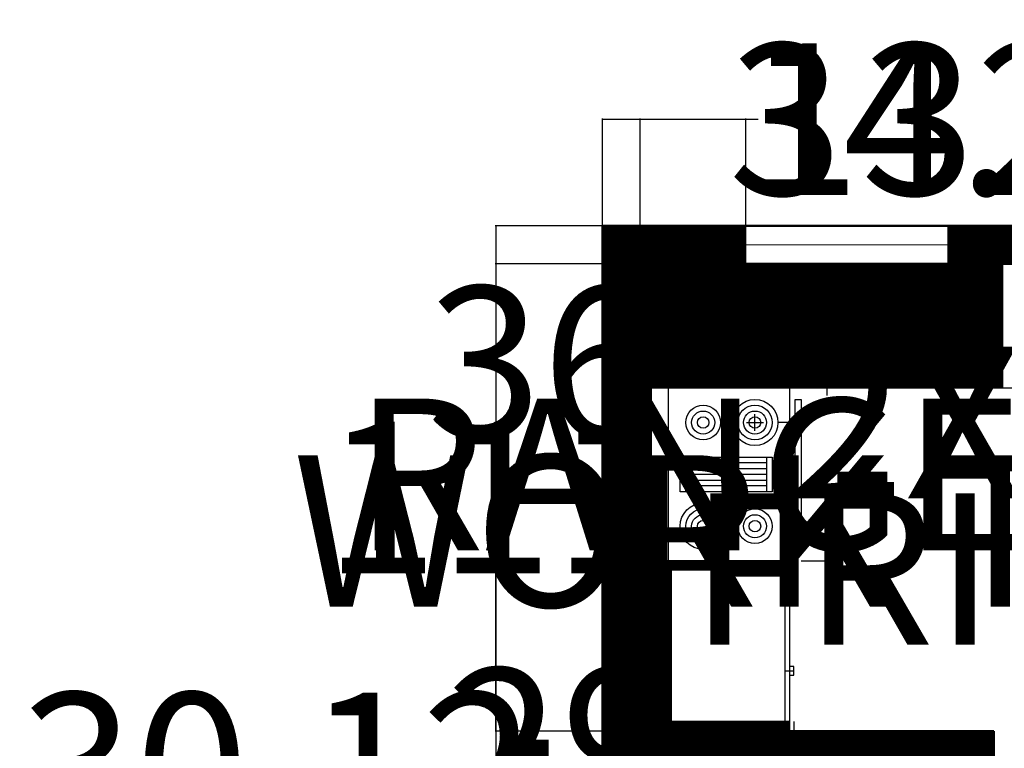
# Model space of a CAD drawing. Units: inches. Extents: x 1173 to 2157, y 515 to 1129.
# Tile 3 of 13: x 1241 to 1475, y 929 to 1102. Entities that reach past the tile are written whole.
import ezdxf

# ---------------------------------------------------------------- set-up
doc = ezdxf.new("R2010")
doc.units = ezdxf.units.IN
doc.header["$MEASUREMENT"] = 0
for name, color, linetype, lineweight in [('A-ANNO-DIMS', 2, 'Continuous', 18), ('A-EQPM', 9, 'Continuous', 25), ('A-FLOR-CASE', 32, 'Continuous', 25), ('A-GLAZ', 4, 'Continuous', 18), ('A-WALL', 7, 'Continuous', 50)]:
    doc.layers.add(name, color=color, linetype=linetype, lineweight=lineweight)
doc.layers.add('A-FLOR-CASE-PATT', color=28, linetype='Continuous', lineweight=13, true_color=0x301203)
doc.layers.add('A-WALL-PATT', color=22, linetype='Continuous', lineweight=13, true_color=0xca4b0c)
doc.styles.get("Standard").update_dxf_attribs({"font": 'arial.ttf'})
doc.dimstyles.get("Standard").update_dxf_attribs({"dimtxt": 36, "dimasz": 0.18, "dimexe": 0.18, "dimexo": 0.0625, "dimgap": 0.09, "dimtad": 0, "dimtih": 1, "dimtoh": 1, "dimdec": 0, "dimrnd": 72, "dimzin": 0, "dimdsep": 46, "dimlunit": 3, "dimtxsty": 'Standard', "dimcen": 2, "dimadec": 0, "dimazin": 0, "dimtfac": 1, "dimtdec": 0, "dimtofl": 0, "dimtmove": 0, "dimatfit": 3, "dimfxl": 1, "dimtolj": 1, "dimtzin": 0, "dimarcsym": 0})

# ---------------------------------------------------------------- blocks, each defined once
blk = doc.blocks.new('Range-Oven - 30 in top')
for p, q in [((0, -3), (30, -3)), ((12, -6), (18, -6)), ((13, -20), (13, -6)), ((14, -6), (14, -20)), ((15, -20), (15, -6)), ((16, -6), (16, -20)), ((17, -20), (17, -6)), ((18, -20), (12, -20)), ((6, -24), (6, -25)), ((8, -25), (8, -24)), ((22, -25), (22, -24)), ((24, -24), (24, -25))]:
    blk.add_line(p, q)
for points in [[(0, -24), (0, 0), (30, 0), (30, -24)], [(12, -21), (12, -5), (18, -5), (18, -21)], [(2, -26), (2, -25), (28, -25), (28, -26)]]:
    blk.add_lwpolyline(points, close=True)
for centre, radius in [((6, -9), 4), ((6, -9), 3), ((24, -9), 3), ((6, -9), 2), ((6, -9), 1), ((24, -9), 2), ((24, -9), 1), ((6, -18), 3), ((24, -18), 4), ((24, -18), 3), ((6, -18), 2), ((6, -18), 1), ((24, -18), 2), ((24, -18), 1)]:
    blk.add_circle(centre, radius)
blk = doc.blocks.new('Refrigerator-2 door - 36 in top')
for p, q in [((0, -26.999999), (36, -26.999999)), ((11, -27.999999), (11, -28.999999)), ((12, -26.999999), (12, -28.999999)), ((13, -28.999999), (13, -27.999999)), ((11, -28.999999), (13, -28.999999))]:
    blk.add_line(p, q)
blk.add_lwpolyline([(0, -27.999999), (0, 0), (36, 0), (36, -27.999999)], close=True)
blk = doc.blocks.new('WIN-48X9')
blk.add_line((48, 4.5), (0, 4.5))
blk.add_lwpolyline([(0, 9), (48, 9), (48, 0), (0, 0)], close=True)
blk = doc.blocks.new('*D36')
at = {"layer": 'A-ANNO-DIMS', "color": 0, "lineweight": -2, "transparency": 16777216}
for p, q in [((1497.87, 905.02), (1487.37, 905.02)), ((1487.55, 904.84), (1487.55, 889.09)), ((1487.55, 835.93), (1487.55, 851.68)), ((1497.87, 835.75), (1487.37, 835.75))]:
    blk.add_line(p, q, dxfattribs=at)
at = {"layer": 'A-ANNO-DIMS', "color": 0, "transparency": 16777216}
for points in [[(1487.52, 904.84), (1487.58, 904.84), (1487.55, 905.02)], [(1487.52, 835.93), (1487.58, 835.93), (1487.55, 835.75)]]:
    blk.add_solid(points, dxfattribs=at)
at = {"layer": 'Defpoints', "color": 0, "transparency": 16777216}
for p in [(1497.94, 905.02), (1487.55, 835.75), (1497.94, 835.75)]:
    blk.add_point(p, dxfattribs=at)
at = {"layer": 'A-ANNO-DIMS', "color": 0, "transparency": 16777216, "insert": (1487.55, 870.38), "char_height": 36, "attachment_point": 5}
blk.add_mtext('\\A1;DINING SET 69', dxfattribs=at)
blk = doc.blocks.new('*D46')
at = {"layer": 'A-ANNO-DIMS', "color": 0, "lineweight": -2, "transparency": 16777216}
for p, q in [((1646.37, 911.98), (1645.86, 896.32)), ((1648.72, 912.09), (1646.2, 912.17)), ((1648.2, 896.07), (1645.68, 896.15)), ((1645.86, 896.14), (1645.85, 895.96)), ((1645.85, 895.96), (1645.67, 895.96))]:
    blk.add_line(p, q, dxfattribs=at)
at = {"layer": 'A-ANNO-DIMS', "color": 0, "transparency": 16777216}
for points in [[(1646.34, 911.99), (1646.4, 911.98), (1646.38, 912.16)], [(1645.83, 896.32), (1645.89, 896.32), (1645.86, 896.14)]]:
    blk.add_solid(points, dxfattribs=at)
at = {"layer": 'Defpoints', "color": 0, "transparency": 16777216}
for p in [(1648.78, 912.09), (1645.86, 896.14), (1648.26, 896.06)]:
    blk.add_point(p, dxfattribs=at)
at = {"layer": 'A-ANNO-DIMS', "color": 0, "transparency": 16777216, "insert": (1538.16, 895.96), "char_height": 36, "attachment_point": 5}
blk.add_mtext('\\A1;BASIN 16', dxfattribs=at)
blk = doc.blocks.new('*D54')
at = {"layer": 'A-ANNO-DIMS', "color": 0, "lineweight": -2, "transparency": 16777216}
for p, q in [((1496.35, 1005.18), (1488.93, 1005.18)), ((1489.11, 1005), (1489.11, 999.54)), ((1489.11, 956.65), (1489.11, 962.11)), ((1496.35, 956.47), (1488.93, 956.47))]:
    blk.add_line(p, q, dxfattribs=at)
at = {"layer": 'A-ANNO-DIMS', "color": 0, "transparency": 16777216}
for points in [[(1489.08, 1005), (1489.14, 1005), (1489.11, 1005.18)], [(1489.08, 956.65), (1489.14, 956.65), (1489.11, 956.47)]]:
    blk.add_solid(points, dxfattribs=at)
at = {"layer": 'Defpoints', "color": 0, "transparency": 16777216}
for p in [(1496.42, 1005.18), (1489.11, 956.47), (1496.42, 956.47)]:
    blk.add_point(p, dxfattribs=at)
at = {"layer": 'A-ANNO-DIMS', "color": 0, "transparency": 16777216, "insert": (1489.11, 980.83), "char_height": 36, "attachment_point": 5}
blk.add_mtext('\\A1;WORK TABLE 49', dxfattribs=at)
blk = doc.blocks.new('*D56')
at = {"layer": 'A-ANNO-DIMS', "color": 0, "lineweight": -2, "transparency": 16777216}
for p, q in [((1426.92, 1014.79), (1433.2, 1014.79)), ((1433.02, 1014.61), (1433.02, 1012.98)), ((1426.92, 973.76), (1433.2, 973.76)), ((1433.02, 973.94), (1433.02, 975.57))]:
    blk.add_line(p, q, dxfattribs=at)
at = {"layer": 'A-ANNO-DIMS', "color": 0, "transparency": 16777216}
for points in [[(1432.99, 1014.61), (1433.05, 1014.61), (1433.02, 1014.79)], [(1432.99, 973.94), (1433.05, 973.94), (1433.02, 973.76)]]:
    blk.add_solid(points, dxfattribs=at)
at = {"layer": 'Defpoints', "color": 0, "transparency": 16777216}
for p in [(1426.86, 1014.79), (1433.02, 1014.79), (1426.86, 973.76)]:
    blk.add_point(p, dxfattribs=at)
at = {"layer": 'A-ANNO-DIMS', "color": 0, "transparency": 16777216, "insert": (1433.02, 994.27), "char_height": 36, "attachment_point": 5}
blk.add_mtext('\\A1;RANGE 41', dxfattribs=at)
blk = doc.blocks.new('*D57')
at = {"layer": 'A-ANNO-DIMS', "color": 0, "lineweight": -2, "transparency": 16777216}
for p, q in [((1391.3, 1020.94), (1391.12, 1020.94)), ((1391.3, 1014.85), (1391.3, 1021.12)), ((1426.68, 1020.94), (1391.48, 1020.94)), ((1426.86, 1014.85), (1426.86, 1021.12))]:
    blk.add_line(p, q, dxfattribs=at)
at = {"layer": 'A-ANNO-DIMS', "color": 0, "transparency": 16777216}
for points in [[(1391.48, 1020.97), (1391.48, 1020.91), (1391.3, 1020.94)], [(1426.68, 1020.97), (1426.68, 1020.91), (1426.86, 1020.94)]]:
    blk.add_solid(points, dxfattribs=at)
at = {"layer": 'Defpoints', "color": 0, "transparency": 16777216}
for p in [(1391.3, 1020.94), (1391.3, 1014.79), (1426.86, 1014.79)]:
    blk.add_point(p, dxfattribs=at)
at = {"layer": 'A-ANNO-DIMS', "color": 0, "transparency": 16777216, "insert": (1365.27, 1020.94), "char_height": 36, "attachment_point": 5}
blk.add_mtext('\\A1;36', dxfattribs=at)
blk = doc.blocks.new('*D60')
at = {"layer": 'A-ANNO-DIMS', "color": 0, "lineweight": -2, "transparency": 16777216}
for p, q in [((1396.06, 971.62), (1390.55, 971.62)), ((1390.73, 971.62), (1390.73, 971.8)), ((1390.73, 971.8), (1390.91, 971.8)), ((1390.73, 935.8), (1390.73, 971.44)), ((1396.06, 935.62), (1390.55, 935.62))]:
    blk.add_line(p, q, dxfattribs=at)
at = {"layer": 'A-ANNO-DIMS', "color": 0, "transparency": 16777216}
for points in [[(1390.7, 971.44), (1390.76, 971.44), (1390.73, 971.62)], [(1390.7, 935.8), (1390.76, 935.8), (1390.73, 935.62)]]:
    blk.add_solid(points, dxfattribs=at)
at = {"layer": 'Defpoints', "color": 0, "transparency": 16777216}
for p in [(1390.73, 971.62), (1396.13, 971.62), (1396.13, 935.62)]:
    blk.add_point(p, dxfattribs=at)
at = {"layer": 'A-ANNO-DIMS', "color": 0, "transparency": 16777216, "insert": (1517.73, 971.8), "char_height": 36, "attachment_point": 5}
blk.add_mtext('\\A1;FRIDGE 36', dxfattribs=at)
blk = doc.blocks.new('*D61')
at = {"layer": 'A-ANNO-DIMS', "color": 0, "lineweight": -2, "transparency": 16777216}
for p, q in [((1396.13, 935.56), (1396.13, 930.04)), ((1425.13, 935.56), (1425.13, 930.04)), ((1396.13, 930.22), (1395.95, 930.22)), ((1424.95, 930.22), (1396.31, 930.22))]:
    blk.add_line(p, q, dxfattribs=at)
at = {"layer": 'A-ANNO-DIMS', "color": 0, "transparency": 16777216}
for points in [[(1396.31, 930.25), (1396.31, 930.19), (1396.13, 930.22)], [(1424.95, 930.25), (1424.95, 930.19), (1425.13, 930.22)]]:
    blk.add_solid(points, dxfattribs=at)
at = {"layer": 'Defpoints', "color": 0, "transparency": 16777216}
for p in [(1396.13, 935.62), (1425.13, 935.62), (1396.13, 930.22)]:
    blk.add_point(p, dxfattribs=at)
at = {"layer": 'A-ANNO-DIMS', "color": 0, "transparency": 16777216, "insert": (1369.73, 930.22), "char_height": 36, "attachment_point": 5}
blk.add_mtext('\\A1;29', dxfattribs=at)
blk = doc.blocks.new('*D65')
at = {"layer": 'A-ANNO-DIMS', "color": 0, "lineweight": -2, "transparency": 16777216}
for p, q in [((1379.6, 1053.28), (1354.18, 1053.28)), ((1354.36, 1053.1), (1354.36, 827.25)), ((1354.36, 564.46), (1354.36, 790.31)), ((1379.6, 564.28), (1354.18, 564.28))]:
    blk.add_line(p, q, dxfattribs=at)
at = {"layer": 'A-ANNO-DIMS', "color": 0, "transparency": 16777216}
for points in [[(1354.33, 1053.1), (1354.39, 1053.1), (1354.36, 1053.28)], [(1354.33, 564.46), (1354.39, 564.46), (1354.36, 564.28)]]:
    blk.add_solid(points, dxfattribs=at)
at = {"layer": 'Defpoints', "color": 0, "transparency": 16777216}
for p in [(1354.36, 1053.28), (1379.66, 1053.28), (1379.66, 564.28)]:
    blk.add_point(p, dxfattribs=at)
at = {"layer": 'A-ANNO-DIMS', "color": 0, "transparency": 16777216, "insert": (1354.36, 808.78), "char_height": 36, "attachment_point": 5}
blk.add_mtext('\\A1;489', dxfattribs=at)
blk = doc.blocks.new('*D66')
at = {"layer": 'A-ANNO-DIMS', "color": 0, "lineweight": -2, "transparency": 16777216}
for p, q in [((1388.6, 1044.28), (1354.18, 1044.28)), ((1354.36, 1044.1), (1354.36, 1006.94)), ((1354.36, 933.46), (1354.36, 970.62)), ((1388.6, 933.28), (1354.18, 933.28))]:
    blk.add_line(p, q, dxfattribs=at)
at = {"layer": 'A-ANNO-DIMS', "color": 0, "transparency": 16777216}
for points in [[(1354.33, 1044.1), (1354.39, 1044.1), (1354.36, 1044.28)], [(1354.33, 933.46), (1354.39, 933.46), (1354.36, 933.28)]]:
    blk.add_solid(points, dxfattribs=at)
at = {"layer": 'Defpoints', "color": 0, "transparency": 16777216}
for p in [(1354.36, 1044.28), (1388.66, 1044.28), (1388.66, 933.28)]:
    blk.add_point(p, dxfattribs=at)
at = {"layer": 'A-ANNO-DIMS', "color": 0, "transparency": 16777216, "insert": (1354.36, 988.78), "char_height": 36, "attachment_point": 5}
blk.add_mtext('\\A1;111', dxfattribs=at)
blk = doc.blocks.new('*D67')
at = {"layer": 'A-ANNO-DIMS', "color": 0, "lineweight": -2, "transparency": 16777216}
for p, q in [((1388.66, 1044.34), (1388.66, 1078.79)), ((1388.84, 1078.61), (1416.68, 1078.61)), ((1520.48, 1078.61), (1492.64, 1078.61)), ((1520.66, 1044.34), (1520.66, 1078.79))]:
    blk.add_line(p, q, dxfattribs=at)
at = {"layer": 'A-ANNO-DIMS', "color": 0, "transparency": 16777216}
for points in [[(1388.84, 1078.64), (1388.84, 1078.58), (1388.66, 1078.61)], [(1520.48, 1078.64), (1520.48, 1078.58), (1520.66, 1078.61)]]:
    blk.add_solid(points, dxfattribs=at)
at = {"layer": 'Defpoints', "color": 0, "transparency": 16777216}
for p in [(1520.66, 1078.61), (1388.66, 1044.28), (1520.66, 1044.28)]:
    blk.add_point(p, dxfattribs=at)
at = {"layer": 'A-ANNO-DIMS', "color": 0, "transparency": 16777216, "insert": (1454.66, 1078.61), "char_height": 36, "attachment_point": 5}
blk.add_mtext('\\A1;132', dxfattribs=at)
blk = doc.blocks.new('*D68')
at = {"layer": 'A-ANNO-DIMS', "color": 0, "lineweight": -2, "transparency": 16777216}
for p, q in [((1379.66, 1053.34), (1379.66, 1078.79)), ((1379.84, 1078.61), (1413.58, 1078.61)), ((1413.76, 1053.34), (1413.76, 1078.79)), ((1413.76, 1078.61), (1413.94, 1078.61))]:
    blk.add_line(p, q, dxfattribs=at)
at = {"layer": 'A-ANNO-DIMS', "color": 0, "transparency": 16777216}
for points in [[(1379.84, 1078.64), (1379.84, 1078.58), (1379.66, 1078.61)], [(1413.58, 1078.64), (1413.58, 1078.58), (1413.76, 1078.61)]]:
    blk.add_solid(points, dxfattribs=at)
at = {"layer": 'Defpoints', "color": 0, "transparency": 16777216}
for p in [(1413.76, 1078.61), (1379.66, 1053.28), (1413.76, 1053.28)]:
    blk.add_point(p, dxfattribs=at)
at = {"layer": 'A-ANNO-DIMS', "color": 0, "transparency": 16777216, "insert": (1457.3, 1078.61), "char_height": 36, "attachment_point": 5}
blk.add_mtext('\\A1;34.1', dxfattribs=at)
blk = doc.blocks.new('*D82')
at = {"layer": 'A-ANNO-DIMS', "color": 0, "lineweight": -2, "transparency": 16777216}
for p, q in [((1363.36, 924.45), (1363.18, 924.45)), ((1388.6, 924.28), (1363.18, 924.27)), ((1363.36, 924.27), (1363.36, 924.45)), ((1363.38, 894.33), (1363.36, 924.09)), ((1388.62, 894.16), (1363.2, 894.15))]:
    blk.add_line(p, q, dxfattribs=at)
at = {"layer": 'A-ANNO-DIMS', "color": 0, "transparency": 16777216}
for points in [[(1363.39, 924.09), (1363.33, 924.09), (1363.36, 924.27)], [(1363.41, 894.33), (1363.35, 894.33), (1363.38, 894.15)]]:
    blk.add_solid(points, dxfattribs=at)
at = {"layer": 'Defpoints', "color": 0, "transparency": 16777216}
for p in [(1363.36, 924.27), (1388.66, 924.28), (1388.68, 894.16)]:
    blk.add_point(p, dxfattribs=at)
at = {"layer": 'A-ANNO-DIMS', "color": 0, "transparency": 16777216, "insert": (1302.55, 924.45), "char_height": 36, "attachment_point": 5}
blk.add_mtext('\\A1;30.12', dxfattribs=at)
blk = doc.blocks.new('*D93')
at = {"layer": 'A-ANNO-DIMS', "color": 0, "lineweight": -2, "transparency": 16777216}
for p, q in [((1473.15, 924.28), (1498.57, 924.28)), ((1498.39, 924.1), (1498.39, 913.61)), ((1473.15, 913.43), (1498.57, 913.43)), ((1498.39, 913.25), (1498.21, 913.25)), ((1498.39, 913.43), (1498.39, 913.25))]:
    blk.add_line(p, q, dxfattribs=at)
at = {"layer": 'A-ANNO-DIMS', "color": 0, "transparency": 16777216}
for points in [[(1498.36, 924.1), (1498.42, 924.1), (1498.39, 924.28)], [(1498.36, 913.61), (1498.42, 913.61), (1498.39, 913.43)]]:
    blk.add_solid(points, dxfattribs=at)
at = {"layer": 'Defpoints', "color": 0, "transparency": 16777216}
for p in [(1473.08, 924.28), (1473.08, 913.43), (1498.39, 913.43)]:
    blk.add_point(p, dxfattribs=at)
at = {"layer": 'A-ANNO-DIMS', "color": 0, "transparency": 16777216, "insert": (1425.05, 913.25), "char_height": 36, "attachment_point": 5}
blk.add_mtext('\\A1;10.848', dxfattribs=at)
blk = doc.blocks.new('*D109')
at = {"layer": 'A-ANNO-DIMS', "color": 0, "lineweight": -2, "transparency": 16777216}
for p, q in [((1638.72, 893.14), (1638.9, 893.14)), ((1638.9, 893.14), (1639.74, 886.91)), ((1641.2, 874.07), (1641.2, 878.07)), ((1639.2, 876.07), (1643.2, 876.07))]:
    blk.add_line(p, q, dxfattribs=at)
at = {"layer": 'A-ANNO-DIMS', "color": 0, "transparency": 16777216}
blk.add_solid([(1639.77, 886.92), (1639.71, 886.91), (1639.77, 886.74)], dxfattribs=at)
at = {"layer": 'Defpoints', "color": 0, "transparency": 16777216}
for p in [(1639.77, 886.74), (1641.2, 876.07)]:
    blk.add_point(p, dxfattribs=at)
at = {"layer": 'A-ANNO-DIMS', "color": 0, "transparency": 16777216, "insert": (1507.71, 893.14), "char_height": 36, "attachment_point": 5}
blk.add_mtext('\\A1;2X R10.766', dxfattribs=at)
blk = doc.blocks.new('*D110')
at = {"layer": 'A-ANNO-DIMS', "color": 0, "lineweight": -2, "transparency": 16777216}
for p, q in [((1415.92, 1004.58), (1415.92, 1008.58)), ((1413.92, 1006.58), (1417.92, 1006.58)), ((1424.67, 1006.58), (1421.57, 1006.58))]:
    blk.add_line(p, q, dxfattribs=at)
at = {"layer": 'A-ANNO-DIMS', "color": 0, "transparency": 16777216}
blk.add_solid([(1421.57, 1006.61), (1421.57, 1006.55), (1421.39, 1006.58)], dxfattribs=at)
at = {"layer": 'Defpoints', "color": 0, "transparency": 16777216}
for p in [(1410.45, 1006.58), (1421.39, 1006.58)]:
    blk.add_point(p, dxfattribs=at)
at = {"layer": 'A-ANNO-DIMS', "color": 0, "transparency": 16777216, "insert": (1556.91, 1006.58), "char_height": 36, "attachment_point": 5}
blk.add_mtext('\\A1;2X ∅10.942', dxfattribs=at)

msp = doc.modelspace()

# ---------------------------------------------------------------- hatches: boundary and pattern name
at = {"layer": 'A-FLOR-CASE-PATT'}
h = msp.add_hatch(dxfattribs=at)
h.set_pattern_fill('ANSI31', color=256)
h.paths.add_polyline_path([(1474.7462, 1044.2805), (1388.6635, 1044.2805), (1388.6635, 1014.7866), (1474.7462, 1014.7866)])
h.paths.add_polyline_path([(1396.1251, 971.618), (1424.1251, 971.618), (1424.1251, 973.7559), (1391.3005, 973.7559), (1391.3005, 1014.7866), (1388.6635, 1014.7866), (1388.6635, 933.2805), (1424.1251, 933.2805), (1424.1251, 935.618), (1396.1251, 935.618)])
at = {"layer": 'A-WALL-PATT'}
h = msp.add_hatch(dxfattribs=at)
h.set_pattern_fill('ANSI31', color=256)
h.paths.add_polyline_path([(1388.6635, 933.2805), (1388.6635, 1044.2805), (1413.7618, 1044.2805), (1413.7618, 1053.2805), (1379.6635, 1053.2805), (1379.6635, 894.1606), (1388.6635, 894.1606), (1388.6635, 924.2805), (1472.6635, 924.2805), (1472.6635, 933.2805)])
h.paths.add_polyline_path([(1520.6635, 1044.2805), (1520.6635, 1014.7866), (1520.6635, 1005.1794), (1520.7714, 1005.1794), (1520.7714, 956.4707), (1520.6635, 924.2805), (1529.6635, 924.2805), (1529.6635, 931.4788), (1529.6635, 1044.2805), (1530.8474, 1044.2805), (1570.9543, 1044.2805), (1570.9543, 1053.2805), (1461.7618, 1053.2805), (1461.7618, 1044.2805)])
h.paths.add_polyline_path([(1618.9543, 1053.2805), (1618.9543, 1044.2805), (1661.6635, 1044.2805), (1661.6635, 1043.7367), (1661.6635, 1032.8874), (1670.6635, 1032.8874), (1670.6635, 1053.2805)])
h.paths.add_polyline_path([(1661.6635, 933.2805), (1661.6635, 927.8377), (1661.6635, 924.2805), (1661.6635, 918.9156), (1670.6635, 918.9156), (1670.6635, 984.8874), (1661.6635, 984.8874), (1661.6635, 978.3712)])
h.paths.add_polyline_path([(1670.6635, 894.9156), (1661.6635, 894.9156), (1661.6635, 890.0349), (1661.9328, 890.0349), (1661.9328, 870.079), (1661.6635, 864.2805), (1589.6635, 864.2805), (1589.6635, 924.2805), (1625.553, 924.2805, -0.02455299), (1625.3782, 927.8377), (1625.3782, 933.2805), (1577.6635, 933.2805), (1577.6635, 924.2805), (1580.6635, 924.2805), (1580.6635, 855.2805), (1586.1062, 855.2805), (1589.6635, 855.2805), (1661.6635, 855.2805), (1661.6635, 826.5597), (1670.6635, 826.5597)])
h.paths.add_polyline_path([(1670.6635, 802.5597), (1661.6635, 802.5597), (1661.6635, 795.2805), (1589.6635, 795.2805), (1589.6635, 819.17, -0.02455299), (1586.1062, 818.9952), (1580.6635, 818.9952), (1580.6635, 795.2805), (1577.6635, 795.2805), (1577.6635, 786.2805), (1661.6635, 786.2805), (1661.6635, 778.5597), (1661.6635, 742.6973), (1670.6635, 742.6973)])
h.paths.add_polyline_path([(1661.6635, 654.2805), (1625.1498, 654.2805), (1625.1498, 645.2805), (1661.3656, 645.2805), (1661.6635, 645.2805), (1661.6635, 573.2805), (1520.6635, 573.2805), (1520.6635, 564.2805), (1670.6635, 564.2805), (1670.6635, 694.6973), (1661.6635, 694.6973)])
h.paths.add_polyline_path([(1529.4367, 733.4702, -0.06854064), (1529.6635, 734.2623), (1529.6635, 795.2805), (1520.6635, 795.2805), (1520.6635, 645.2805), (1577.1498, 645.2805), (1577.1498, 654.2805), (1529.6635, 654.2805), (1529.6635, 686.5626, -0.06854064), (1529.4367, 687.3547)])
h.paths.add_polyline_path([(1379.6635, 711.2805), (1388.6635, 711.2805), (1458.7214, 711.2805), (1458.7214, 720.2805), (1410.7214, 720.2805), (1388.6635, 720.2805), (1388.6635, 745.0427), (1379.6635, 745.0427)])
h.paths.add_polyline_path([(1388.6635, 846.1606), (1379.6635, 846.1606), (1379.6635, 793.0427), (1388.6635, 793.0427)])

# ---------------------------------------------------------------- linework, layer by layer
at = {"layer": 'A-FLOR-CASE'}
for p, q in [((1388.6635, 1044.2805), (1430.6635, 1044.2805)), ((1388.6635, 933.2805), (1388.6635, 1044.2805)), ((1424.1251, 1014.7866), (1424.1251, 933.2805)), ((1430.6635, 933.2805), (1388.6635, 933.2805))]:
    msp.add_line(p, q, dxfattribs=at)
msp.add_lwpolyline([(1424.1251, 1014.7866), (1520.6635, 1014.7866), (1520.6635, 1044.2805), (1388.6635, 1044.2805), (1388.6635, 1014.7866)], dxfattribs=at)
msp.add_lwpolyline([(1388.6635, 1044.2805), (1474.7462, 1044.2805), (1474.7462, 1014.7866), (1388.6635, 1014.7866)], close=True, dxfattribs=at)
at = {"layer": 'A-WALL'}
for p, q in [((1388.6635, 1044.2805), (1388.6635, 933.2805)), ((1520.6635, 1044.2805), (1388.6635, 1044.2805)), ((1472.6635, 933.2805), (1388.6635, 933.2805)), ((1472.6635, 924.2805), (1472.6635, 933.2805))]:
    msp.add_line(p, q, dxfattribs=at)
msp.add_lwpolyline([(1379.6635, 564.2805), (1670.6635, 564.2805), (1670.6635, 1053.2805), (1379.6635, 1053.2805)], close=True, dxfattribs=at)

# ---------------------------------------------------------------- block references
at = {"layer": 'A-EQPM', "xscale": 1.36769001067488, "yscale": 1.36769001067488, "zscale": 1.36769001067488, "rotation": 90}
msp.add_blockref('Range-Oven - 30 in top', (1391.3005, 973.7559), dxfattribs=at)
at = {"layer": 'A-EQPM', "rotation": 90}
msp.add_blockref('Refrigerator-2 door - 36 in top', (1396.1251, 935.618), dxfattribs=at)
at = {"layer": 'A-GLAZ'}
msp.add_blockref('WIN-48X9', (1413.7618, 1044.2805), dxfattribs=at)

# ---------------------------------------------------------------- dimensions: what is measured, and where the dimension line sits
at = {"layer": 'A-ANNO-DIMS'}
for base, p1, p2, override, picture, middle in [((1413.7618, 1078.6127), (1379.6635, 1053.2805), (1413.7618, 1053.2805), {"dimdec": 1, "dimlfac": 1, "dimrnd": 0, "dimzin": 0, "dimdsep": 46, "dimlunit": 2}, '*D68', (1457.3006, 1078.6127)), ((1520.6635, 1078.6127), (1388.6635, 1044.2805), (1520.6635, 1044.2805), {"dimdec": 0, "dimlfac": 1, "dimrnd": 0, "dimzin": 0, "dimdsep": 46, "dimlunit": 2}, '*D67', (1454.6635, 1078.6127))]:
    dim = msp.add_linear_dim(base=base, p1=p1, p2=p2, dimstyle='Standard', override=override, dxfattribs=at)
    dim.commit()
    dim.dimension.update_dxf_attribs({"geometry": picture, "text_midpoint": middle})
for base, p1, p2, angle, text, picture, middle in [((1489.1107, 956.4707), (1496.4171, 1005.1794), (1496.4171, 956.4707), 270, 'WORK TABLE <>', '*D54', (1489.1107, 980.8251)), ((1433.0151, 1014.7866), (1426.8605, 973.7559), (1426.8605, 1014.7866), 90, 'RANGE <>', '*D56', (1433.0151, 994.2712)), ((1390.7251, 971.618), (1396.1251, 935.618), (1396.1251, 971.618), 90, 'FRIDGE <>', '*D60', (1517.7318, 971.798)), ((1487.5464, 835.7486), (1497.9367, 905.017), (1497.9367, 835.7486), 270, 'DINING SET <>', '*D36', (1487.5464, 870.3828)), ((1645.8589, 896.1412), (1648.7786, 912.0868), (1648.2623, 896.0638), 268.15447, 'BASIN <>', '*D46', (1538.1601, 895.9613))]:
    dim = msp.add_linear_dim(base=base, p1=p1, p2=p2, angle=angle, text=text, dimstyle='Standard', override={"dimdec": 0, "dimlfac": 1, "dimrnd": 0, "dimzin": 0, "dimdsep": 46, "dimlunit": 2}, dxfattribs=at)
    dim.commit()
    dim.dimension.update_dxf_attribs({"geometry": picture, "text_midpoint": middle})
dim = msp.add_diameter_dim_2p(p1=(1410.4482, 1006.5809), p2=(1421.3897, 1006.58), text='2X <>', dimstyle='Standard', override={"dimdec": 3, "dimlfac": 1, "dimrnd": 0, "dimzin": 0, "dimdsep": 46, "dimlunit": 2}, dxfattribs=at)
dim.commit()
dim.dimension.update_dxf_attribs({"geometry": '*D110', "text_midpoint": (1424.6722, 1006.5797), "dimtype": 163})
for base, p1, p2, angle, override, picture, middle in [((1354.361, 1053.2805), (1379.6635, 564.2805), (1379.6635, 1053.2805), 90, {"dimdec": 0, "dimlfac": 1, "dimrnd": 0, "dimzin": 0, "dimdsep": 46, "dimlunit": 2}, '*D65', (1354.361, 808.7805)), ((1354.361, 1044.2805), (1388.6635, 933.2805), (1388.6635, 1044.2805), 90, {"dimdec": 0, "dimlfac": 1, "dimrnd": 0, "dimzin": 0, "dimdsep": 46, "dimlunit": 2}, '*D66', (1354.361, 988.7805)), ((1391.3005, 1020.9412), (1426.8605, 1014.7866), (1391.3005, 1014.7866), 180, {"dimdec": 0, "dimlfac": 1, "dimrnd": 0, "dimzin": 0, "dimdsep": 46, "dimlunit": 2}, '*D57', (1365.2706, 1020.9412)), ((1396.1251, 930.218), (1425.1251, 935.618), (1396.1251, 935.618), 180, {"dimdec": 0, "dimlfac": 1, "dimrnd": 0, "dimzin": 0, "dimdsep": 46, "dimlunit": 2}, '*D61', (1369.7269, 930.218)), ((1363.361, 924.268), (1388.6784, 894.1606), (1388.6635, 924.2805), 90.028445, {"dimdec": 2, "dimlfac": 1, "dimrnd": 0, "dimzin": 0, "dimdsep": 46, "dimlunit": 2}, '*D82', (1302.5465, 924.448)), ((1498.3865, 913.4324), (1473.084, 924.2805), (1473.084, 913.4324), 270, {"dimdec": 3, "dimlfac": 1, "dimrnd": 0, "dimzin": 0, "dimdsep": 46, "dimlunit": 2}, '*D93', (1425.0483, 913.2524))]:
    dim = msp.add_linear_dim(base=base, p1=p1, p2=p2, angle=angle, dimstyle='Standard', override=override, dxfattribs=at)
    dim.commit()
    dim.dimension.update_dxf_attribs({"geometry": picture, "text_midpoint": middle})
dim = msp.add_radius_dim(center=(1641.2, 876.0658), mpoint=(1639.765, 886.7357), text='2X <>', dimstyle='Standard', override={"dimdec": 3, "dimlfac": 1, "dimrnd": 0, "dimzin": 0, "dimdsep": 46, "dimlunit": 2}, dxfattribs=at)
dim.commit()
dim.dimension.update_dxf_attribs({"geometry": '*D109', "text_midpoint": (1507.7105, 893.1376), "dimtype": 164})

doc.saveas('drawing.dxf')
